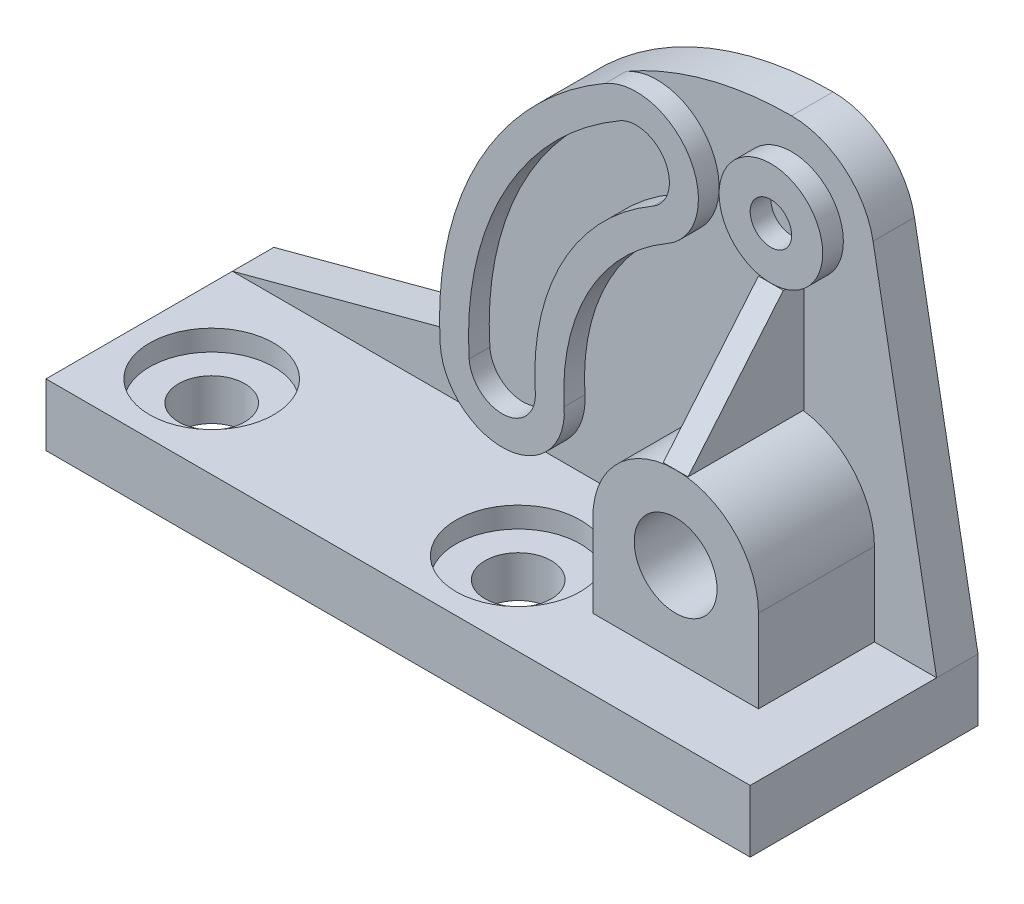
ISO-10303-21;
HEADER;
FILE_DESCRIPTION(('STEP AP214'),'2;1');
FILE_NAME('part.step','',(''),(''),'','','');
FILE_SCHEMA(('AUTOMOTIVE_DESIGN { 1 0 10303 214 1 1 1 1 }'));
ENDSEC;
DATA;
#1=APPLICATION_CONTEXT('core data for automotive mechanical design processes');
#2=APPLICATION_PROTOCOL_DEFINITION('international standard','automotive_design',2000,#1);
#3=PRODUCT_CONTEXT('',#1,'mechanical');
#4=PRODUCT('Part','Part','',(#3));
#5=PRODUCT_RELATED_PRODUCT_CATEGORY('part','',(#4));
#6=PRODUCT_DEFINITION_FORMATION('','',#4);
#7=PRODUCT_DEFINITION_CONTEXT('part definition',#1,'design');
#8=PRODUCT_DEFINITION('design','',#6,#7);
#9=PRODUCT_DEFINITION_SHAPE('','',#8);
#10=(LENGTH_UNIT() NAMED_UNIT(*) SI_UNIT(.MILLI.,.METRE.));
#11=(NAMED_UNIT(*) PLANE_ANGLE_UNIT() SI_UNIT($,.RADIAN.));
#12=(NAMED_UNIT(*) SI_UNIT($,.STERADIAN.) SOLID_ANGLE_UNIT());
#13=UNCERTAINTY_MEASURE_WITH_UNIT(LENGTH_MEASURE(1.E-05),#10,'distance_accuracy_value','');
#14=(GEOMETRIC_REPRESENTATION_CONTEXT(3) GLOBAL_UNCERTAINTY_ASSIGNED_CONTEXT((#13)) GLOBAL_UNIT_ASSIGNED_CONTEXT((#10,
#11,#12)) REPRESENTATION_CONTEXT('',''));
#15=CARTESIAN_POINT('',(0.,0.,0.));
#16=DIRECTION('',(0.,0.,1.));
#17=DIRECTION('',(1.,0.,0.));
#18=AXIS2_PLACEMENT_3D('',#15,#16,#17);
#19=CARTESIAN_POINT('',(26.5,41.25,-6.25));
#20=DIRECTION('',(0.,-1.,0.));
#21=DIRECTION('',(0.,0.,-1.));
#22=AXIS2_PLACEMENT_3D('',#19,#20,#21);
#23=PLANE('',#22);
#24=DIRECTION('',(0.,0.,1.));
#25=VECTOR('',#24,1.);
#26=CARTESIAN_POINT('',(23.5,41.25,-6.25));
#27=LINE('',#26,#25);
#28=CARTESIAN_POINT('',(23.5,41.25,-8.75));
#29=VERTEX_POINT('',#28);
#30=CARTESIAN_POINT('',(23.5,41.25,-6.25));
#31=VERTEX_POINT('',#30);
#32=EDGE_CURVE('E115',#29,#31,#27,.T.);
#33=ORIENTED_EDGE('',*,*,#32,.T.);
#34=DIRECTION('',(-1.,0.,0.));
#35=VECTOR('',#34,1.);
#36=CARTESIAN_POINT('',(26.5,41.25,-6.25));
#37=LINE('',#36,#35);
#38=CARTESIAN_POINT('',(26.5,41.25,-6.25));
#39=VERTEX_POINT('',#38);
#40=EDGE_CURVE('E12',#39,#31,#37,.T.);
#41=ORIENTED_EDGE('',*,*,#40,.F.);
#42=DIRECTION('',(0.,0.,1.));
#43=VECTOR('',#42,1.);
#44=CARTESIAN_POINT('',(26.5,41.25,-6.25));
#45=LINE('',#44,#43);
#46=CARTESIAN_POINT('',(26.5,41.25,-8.75));
#47=VERTEX_POINT('',#46);
#48=EDGE_CURVE('E99',#47,#39,#45,.T.);
#49=ORIENTED_EDGE('',*,*,#48,.F.);
#50=DIRECTION('',(-1.,0.,0.));
#51=VECTOR('',#50,1.);
#52=CARTESIAN_POINT('',(26.5,41.25,-8.75));
#53=LINE('',#52,#51);
#54=EDGE_CURVE('E107',#47,#29,#53,.T.);
#55=ORIENTED_EDGE('',*,*,#54,.T.);
#56=EDGE_LOOP('',(#33,#41,#49,#55));
#57=FACE_BOUND('',#56,.T.);
#58=ADVANCED_FACE('F47',(#57),#23,.F.);
#59=CARTESIAN_POINT('',(26.5,41.25,-6.25));
#60=DIRECTION('',(0.,-0.641555200491106,-0.767076870152409));
#61=DIRECTION('',(0.,0.767076870152409,-0.641555200491106));
#62=AXIS2_PLACEMENT_3D('',#59,#60,#61);
#63=PLANE('',#62);
#64=DIRECTION('',(0.,-0.767076870152409,0.641555200491106));
#65=VECTOR('',#64,1.);
#66=CARTESIAN_POINT('',(23.5,41.25,-6.25));
#67=LINE('',#66,#65);
#68=CARTESIAN_POINT('',(23.5,27.5,5.25));
#69=VERTEX_POINT('',#68);
#70=EDGE_CURVE('E102',#31,#69,#67,.T.);
#71=ORIENTED_EDGE('',*,*,#70,.T.);
#72=DIRECTION('',(-1.,0.,0.));
#73=VECTOR('',#72,1.);
#74=CARTESIAN_POINT('',(26.5,27.5,5.25));
#75=LINE('',#74,#73);
#76=CARTESIAN_POINT('',(26.5,27.5,5.25));
#77=VERTEX_POINT('',#76);
#78=EDGE_CURVE('E60',#77,#69,#75,.T.);
#79=ORIENTED_EDGE('',*,*,#78,.F.);
#80=DIRECTION('',(0.,-0.767076870152409,0.641555200491106));
#81=VECTOR('',#80,1.);
#82=CARTESIAN_POINT('',(26.5,41.25,-6.25));
#83=LINE('',#82,#81);
#84=EDGE_CURVE('E92',#39,#77,#83,.T.);
#85=ORIENTED_EDGE('',*,*,#84,.F.);
#86=ORIENTED_EDGE('',*,*,#40,.T.);
#87=EDGE_LOOP('',(#71,#79,#85,#86));
#88=FACE_BOUND('',#87,.T.);
#89=ADVANCED_FACE('F103',(#88),#63,.F.);
#90=CARTESIAN_POINT('',(26.5,27.5,-8.75));
#91=DIRECTION('',(0.,1.,0.));
#92=DIRECTION('',(0.,0.,1.));
#93=AXIS2_PLACEMENT_3D('',#90,#91,#92);
#94=PLANE('',#93);
#95=DIRECTION('',(0.,0.,-1.));
#96=VECTOR('',#95,1.);
#97=CARTESIAN_POINT('',(23.5,27.5,-8.75));
#98=LINE('',#97,#96);
#99=CARTESIAN_POINT('',(23.5,27.5,-8.75));
#100=VERTEX_POINT('',#99);
#101=EDGE_CURVE('E85',#69,#100,#98,.T.);
#102=ORIENTED_EDGE('',*,*,#101,.T.);
#103=DIRECTION('',(-1.,0.,0.));
#104=VECTOR('',#103,1.);
#105=CARTESIAN_POINT('',(26.5,27.5,-8.75));
#106=LINE('',#105,#104);
#107=CARTESIAN_POINT('',(26.5,27.5,-8.75));
#108=VERTEX_POINT('',#107);
#109=EDGE_CURVE('E104',#108,#100,#106,.T.);
#110=ORIENTED_EDGE('',*,*,#109,.F.);
#111=DIRECTION('',(0.,0.,-1.));
#112=VECTOR('',#111,1.);
#113=CARTESIAN_POINT('',(26.5,27.5,-8.75));
#114=LINE('',#113,#112);
#115=EDGE_CURVE('E98',#77,#108,#114,.T.);
#116=ORIENTED_EDGE('',*,*,#115,.F.);
#117=ORIENTED_EDGE('',*,*,#78,.T.);
#118=EDGE_LOOP('',(#102,#110,#116,#117));
#119=FACE_BOUND('',#118,.T.);
#120=ADVANCED_FACE('F106',(#119),#94,.F.);
#121=CARTESIAN_POINT('',(26.5,41.25,-8.75));
#122=DIRECTION('',(0.,0.,1.));
#123=DIRECTION('',(1.,0.,0.));
#124=AXIS2_PLACEMENT_3D('',#121,#122,#123);
#125=PLANE('',#124);
#126=DIRECTION('',(0.,1.,0.));
#127=VECTOR('',#126,1.);
#128=CARTESIAN_POINT('',(23.5,41.25,-8.75));
#129=LINE('',#128,#127);
#130=EDGE_CURVE('E86',#100,#29,#129,.T.);
#131=ORIENTED_EDGE('',*,*,#130,.T.);
#132=ORIENTED_EDGE('',*,*,#54,.F.);
#133=DIRECTION('',(0.,1.,0.));
#134=VECTOR('',#133,1.);
#135=CARTESIAN_POINT('',(26.5,41.25,-8.75));
#136=LINE('',#135,#134);
#137=EDGE_CURVE('E65',#108,#47,#136,.T.);
#138=ORIENTED_EDGE('',*,*,#137,.F.);
#139=ORIENTED_EDGE('',*,*,#109,.T.);
#140=EDGE_LOOP('',(#131,#132,#138,#139));
#141=FACE_BOUND('',#140,.T.);
#142=ADVANCED_FACE('F118',(#141),#125,.F.);
#143=CARTESIAN_POINT('',(26.5,0.,0.));
#144=DIRECTION('',(-1.,0.,0.));
#145=DIRECTION('',(0.,0.,1.));
#146=AXIS2_PLACEMENT_3D('',#143,#144,#145);
#147=PLANE('',#146);
#148=ORIENTED_EDGE('',*,*,#48,.T.);
#149=ORIENTED_EDGE('',*,*,#84,.T.);
#150=ORIENTED_EDGE('',*,*,#115,.T.);
#151=ORIENTED_EDGE('',*,*,#137,.T.);
#152=EDGE_LOOP('',(#148,#149,#150,#151));
#153=FACE_BOUND('',#152,.T.);
#154=ADVANCED_FACE('F96',(#153),#147,.F.);
#155=CARTESIAN_POINT('',(23.5,0.,0.));
#156=DIRECTION('',(-1.,0.,0.));
#157=DIRECTION('',(0.,0.,1.));
#158=AXIS2_PLACEMENT_3D('',#155,#156,#157);
#159=PLANE('',#158);
#160=ORIENTED_EDGE('',*,*,#32,.F.);
#161=ORIENTED_EDGE('',*,*,#130,.F.);
#162=ORIENTED_EDGE('',*,*,#101,.F.);
#163=ORIENTED_EDGE('',*,*,#70,.F.);
#164=EDGE_LOOP('',(#160,#161,#162,#163));
#165=FACE_BOUND('',#164,.T.);
#166=ADVANCED_FACE('F125',(#165),#159,.T.);
#167=CLOSED_SHELL('',(#58,#89,#120,#142,#154,#166));
#168=MANIFOLD_SOLID_BREP('B2',#167);
#169=CARTESIAN_POINT('',(25.,17.5,-8.75));
#170=DIRECTION('',(0.,0.,1.));
#171=DIRECTION('',(1.,0.,0.));
#172=AXIS2_PLACEMENT_3D('',#169,#170,#171);
#173=PLANE('',#172);
#174=CARTESIAN_POINT('',(25.,47.5,-8.75));
#175=DIRECTION('',(0.,0.,1.));
#176=DIRECTION('',(1.,0.,0.));
#177=AXIS2_PLACEMENT_3D('',#174,#175,#176);
#178=CIRCLE('',#177,6.25);
#179=CARTESIAN_POINT('',(31.25,47.5,-8.75));
#180=VERTEX_POINT('',#179);
#181=EDGE_CURVE('E430',#180,#180,#178,.T.);
#182=ORIENTED_EDGE('',*,*,#181,.F.);
#183=EDGE_LOOP('',(#182));
#184=FACE_BOUND('',#183,.T.);
#185=CARTESIAN_POINT('',(25.,17.5,-8.75));
#186=DIRECTION('',(0.,0.,-1.));
#187=DIRECTION('',(1.,0.,0.));
#188=AXIS2_PLACEMENT_3D('',#185,#186,#187);
#189=CIRCLE('',#188,40.);
#190=CARTESIAN_POINT('',(5.00000000000002,52.1410161513775,-8.75));
#191=VERTEX_POINT('',#190);
#192=CARTESIAN_POINT('',(25.,57.5,-8.75));
#193=VERTEX_POINT('',#192);
#194=EDGE_CURVE('E432',#191,#193,#189,.T.);
#195=ORIENTED_EDGE('',*,*,#194,.F.);
#196=CARTESIAN_POINT('',(8.74999999999999,45.6458256229943,-8.75));
#197=DIRECTION('',(0.,0.,1.));
#198=DIRECTION('',(-1.,0.,0.));
#199=AXIS2_PLACEMENT_3D('',#196,#197,#198);
#200=CIRCLE('',#199,7.49999999999999);
#201=CARTESIAN_POINT('',(12.5,39.1506350946109,-8.75));
#202=VERTEX_POINT('',#201);
#203=EDGE_CURVE('E326',#202,#191,#200,.T.);
#204=ORIENTED_EDGE('',*,*,#203,.F.);
#205=CARTESIAN_POINT('',(25.,17.5,-8.75));
#206=DIRECTION('',(0.,0.,-1.));
#207=DIRECTION('',(1.,0.,0.));
#208=AXIS2_PLACEMENT_3D('',#205,#206,#207);
#209=CIRCLE('',#208,25.);
#210=CARTESIAN_POINT('',(0.0532183429704687,15.8696365569313,-8.75));
#211=VERTEX_POINT('',#210);
#212=EDGE_CURVE('E352',#211,#202,#209,.T.);
#213=ORIENTED_EDGE('',*,*,#212,.F.);
#214=CARTESIAN_POINT('',(-7.4308161541384,15.3805275240106,-8.75));
#215=DIRECTION('',(0.,0.,1.));
#216=DIRECTION('',(1.,0.,0.));
#217=AXIS2_PLACEMENT_3D('',#214,#215,#216);
#218=CIRCLE('',#217,7.5);
#219=CARTESIAN_POINT('',(-14.9148506512472,14.89141849109,-8.75));
#220=VERTEX_POINT('',#219);
#221=EDGE_CURVE('E363',#220,#211,#218,.T.);
#222=ORIENTED_EDGE('',*,*,#221,.F.);
#223=DIRECTION('',(0.96592582628907,0.258819045102514,0.));
#224=VECTOR('',#223,1.);
#225=CARTESIAN_POINT('',(-42.5,7.5,-8.75));
#226=LINE('',#225,#224);
#227=CARTESIAN_POINT('',(-42.5,7.5,-8.75));
#228=VERTEX_POINT('',#227);
#229=EDGE_CURVE('E447',#228,#220,#226,.T.);
#230=ORIENTED_EDGE('',*,*,#229,.F.);
#231=DIRECTION('',(-1.,0.,0.));
#232=VECTOR('',#231,1.);
#233=CARTESIAN_POINT('',(42.5,7.5,-8.75));
#234=LINE('',#233,#232);
#235=CARTESIAN_POINT('',(15.,7.5,-8.75));
#236=VERTEX_POINT('',#235);
#237=EDGE_CURVE('E444',#236,#228,#234,.T.);
#238=ORIENTED_EDGE('',*,*,#237,.F.);
#239=DIRECTION('',(0.,-1.,0.));
#240=VECTOR('',#239,1.);
#241=CARTESIAN_POINT('',(15.,17.5,-8.75));
#242=LINE('',#241,#240);
#243=CARTESIAN_POINT('',(15.,17.5,-8.75));
#244=VERTEX_POINT('',#243);
#245=EDGE_CURVE('E415',#244,#236,#242,.T.);
#246=ORIENTED_EDGE('',*,*,#245,.F.);
#247=CARTESIAN_POINT('',(25.,17.5,-8.75));
#248=DIRECTION('',(0.,0.,1.));
#249=DIRECTION('',(1.,0.,0.));
#250=AXIS2_PLACEMENT_3D('',#247,#248,#249);
#251=CIRCLE('',#250,10.);
#252=CARTESIAN_POINT('',(35.,17.5,-8.75));
#253=VERTEX_POINT('',#252);
#254=EDGE_CURVE('E397',#253,#244,#251,.T.);
#255=ORIENTED_EDGE('',*,*,#254,.F.);
#256=DIRECTION('',(0.,1.,0.));
#257=VECTOR('',#256,1.);
#258=CARTESIAN_POINT('',(35.,7.5,-8.75));
#259=LINE('',#258,#257);
#260=CARTESIAN_POINT('',(35.,7.5,-8.75));
#261=VERTEX_POINT('',#260);
#262=EDGE_CURVE('E401',#261,#253,#259,.T.);
#263=ORIENTED_EDGE('',*,*,#262,.F.);
#264=CARTESIAN_POINT('',(42.5,7.5,-8.75));
#265=VERTEX_POINT('',#264);
#266=EDGE_CURVE('E441',#265,#261,#234,.T.);
#267=ORIENTED_EDGE('',*,*,#266,.F.);
#268=DIRECTION('',(0.180327868852459,-0.983606557377049,0.));
#269=VECTOR('',#268,1.);
#270=CARTESIAN_POINT('',(34.8360655737705,49.3032786885246,-8.75));
#271=LINE('',#270,#269);
#272=CARTESIAN_POINT('',(34.8360655737705,49.3032786885246,-8.75));
#273=VERTEX_POINT('',#272);
#274=EDGE_CURVE('E439',#273,#265,#271,.T.);
#275=ORIENTED_EDGE('',*,*,#274,.F.);
#276=CARTESIAN_POINT('',(25.,47.5,-8.75));
#277=DIRECTION('',(0.,0.,-1.));
#278=DIRECTION('',(-1.,0.,0.));
#279=AXIS2_PLACEMENT_3D('',#276,#277,#278);
#280=CIRCLE('',#279,10.);
#281=EDGE_CURVE('E436',#193,#273,#280,.T.);
#282=ORIENTED_EDGE('',*,*,#281,.F.);
#283=EDGE_LOOP('',(#195,#204,#213,#222,#230,#238,#246,#255,#263,#267,#275,#282));
#284=FACE_BOUND('',#283,.T.);
#285=ADVANCED_FACE('F174',(#184,#284),#173,.T.);
#286=CARTESIAN_POINT('',(0.,7.5,0.));
#287=DIRECTION('',(0.,-1.,0.));
#288=DIRECTION('',(0.,0.,-1.));
#289=AXIS2_PLACEMENT_3D('',#286,#287,#288);
#290=PLANE('',#289);
#291=CARTESIAN_POINT('',(4.5,7.5,3.75));
#292=DIRECTION('',(0.,1.,0.));
#293=DIRECTION('',(0.,0.,1.));
#294=AXIS2_PLACEMENT_3D('',#291,#292,#293);
#295=CIRCLE('',#294,7.5);
#296=CARTESIAN_POINT('',(4.5,7.5,11.25));
#297=VERTEX_POINT('',#296);
#298=EDGE_CURVE('E389',#297,#297,#295,.T.);
#299=ORIENTED_EDGE('',*,*,#298,.F.);
#300=EDGE_LOOP('',(#299));
#301=FACE_BOUND('',#300,.T.);
#302=CARTESIAN_POINT('',(-32.5,7.5,3.75));
#303=DIRECTION('',(0.,1.,0.));
#304=DIRECTION('',(0.,0.,1.));
#305=AXIS2_PLACEMENT_3D('',#302,#303,#304);
#306=CIRCLE('',#305,7.5);
#307=CARTESIAN_POINT('',(-32.5,7.5,11.25));
#308=VERTEX_POINT('',#307);
#309=EDGE_CURVE('E374',#308,#308,#306,.T.);
#310=ORIENTED_EDGE('',*,*,#309,.F.);
#311=EDGE_LOOP('',(#310));
#312=FACE_BOUND('',#311,.T.);
#313=DIRECTION('',(0.,0.,-1.));
#314=VECTOR('',#313,1.);
#315=CARTESIAN_POINT('',(15.,7.5,5.25));
#316=LINE('',#315,#314);
#317=CARTESIAN_POINT('',(15.,7.5,5.25));
#318=VERTEX_POINT('',#317);
#319=EDGE_CURVE('E420',#318,#236,#316,.T.);
#320=ORIENTED_EDGE('',*,*,#319,.T.);
#321=ORIENTED_EDGE('',*,*,#237,.T.);
#322=DIRECTION('',(0.,0.,1.));
#323=VECTOR('',#322,1.);
#324=CARTESIAN_POINT('',(-42.5,7.5,13.75));
#325=LINE('',#324,#323);
#326=CARTESIAN_POINT('',(-42.5,7.5,13.75));
#327=VERTEX_POINT('',#326);
#328=EDGE_CURVE('E472',#228,#327,#325,.T.);
#329=ORIENTED_EDGE('',*,*,#328,.T.);
#330=DIRECTION('',(1.,0.,0.));
#331=VECTOR('',#330,1.);
#332=CARTESIAN_POINT('',(-42.5,7.5,13.75));
#333=LINE('',#332,#331);
#334=CARTESIAN_POINT('',(42.5,7.5,13.75));
#335=VERTEX_POINT('',#334);
#336=EDGE_CURVE('E480',#327,#335,#333,.T.);
#337=ORIENTED_EDGE('',*,*,#336,.T.);
#338=DIRECTION('',(0.,0.,-1.));
#339=VECTOR('',#338,1.);
#340=CARTESIAN_POINT('',(42.5,7.5,13.75));
#341=LINE('',#340,#339);
#342=EDGE_CURVE('E468',#335,#265,#341,.T.);
#343=ORIENTED_EDGE('',*,*,#342,.T.);
#344=ORIENTED_EDGE('',*,*,#266,.T.);
#345=DIRECTION('',(0.,0.,-1.));
#346=VECTOR('',#345,1.);
#347=CARTESIAN_POINT('',(35.,7.5,5.25));
#348=LINE('',#347,#346);
#349=CARTESIAN_POINT('',(35.,7.5,5.25));
#350=VERTEX_POINT('',#349);
#351=EDGE_CURVE('E417',#350,#261,#348,.T.);
#352=ORIENTED_EDGE('',*,*,#351,.F.);
#353=DIRECTION('',(1.,0.,0.));
#354=VECTOR('',#353,1.);
#355=CARTESIAN_POINT('',(15.,7.5,5.25));
#356=LINE('',#355,#354);
#357=EDGE_CURVE('E403',#318,#350,#356,.T.);
#358=ORIENTED_EDGE('',*,*,#357,.F.);
#359=EDGE_LOOP('',(#320,#321,#329,#337,#343,#344,#352,#358));
#360=FACE_BOUND('',#359,.T.);
#361=ADVANCED_FACE('F527',(#301,#312,#360),#290,.F.);
#362=CARTESIAN_POINT('',(42.5,7.5,13.75));
#363=DIRECTION('',(-1.,0.,0.));
#364=DIRECTION('',(0.,0.,1.));
#365=AXIS2_PLACEMENT_3D('',#362,#363,#364);
#366=PLANE('',#365);
#367=DIRECTION('',(0.,0.,-1.));
#368=VECTOR('',#367,1.);
#369=CARTESIAN_POINT('',(42.5,0.,13.75));
#370=LINE('',#369,#368);
#371=CARTESIAN_POINT('',(42.5,0.,13.75));
#372=VERTEX_POINT('',#371);
#373=CARTESIAN_POINT('',(42.5,0.,-13.75));
#374=VERTEX_POINT('',#373);
#375=EDGE_CURVE('E464',#372,#374,#370,.T.);
#376=ORIENTED_EDGE('',*,*,#375,.T.);
#377=DIRECTION('',(0.,-1.,0.));
#378=VECTOR('',#377,1.);
#379=CARTESIAN_POINT('',(42.5,7.5,-13.75));
#380=LINE('',#379,#378);
#381=CARTESIAN_POINT('',(42.5,7.5,-13.75));
#382=VERTEX_POINT('',#381);
#383=EDGE_CURVE('E494',#382,#374,#380,.T.);
#384=ORIENTED_EDGE('',*,*,#383,.F.);
#385=DIRECTION('',(0.,0.,-1.));
#386=VECTOR('',#385,1.);
#387=CARTESIAN_POINT('',(42.5,7.5,-8.75));
#388=LINE('',#387,#386);
#389=EDGE_CURVE('E463',#265,#382,#388,.T.);
#390=ORIENTED_EDGE('',*,*,#389,.F.);
#391=ORIENTED_EDGE('',*,*,#342,.F.);
#392=DIRECTION('',(0.,-1.,0.));
#393=VECTOR('',#392,1.);
#394=CARTESIAN_POINT('',(42.5,7.5,13.75));
#395=LINE('',#394,#393);
#396=EDGE_CURVE('E479',#335,#372,#395,.T.);
#397=ORIENTED_EDGE('',*,*,#396,.T.);
#398=EDGE_LOOP('',(#376,#384,#390,#391,#397));
#399=FACE_BOUND('',#398,.T.);
#400=ADVANCED_FACE('F175',(#399),#366,.F.);
#401=CARTESIAN_POINT('',(-42.5,7.5,-13.75));
#402=DIRECTION('',(0.,0.,1.));
#403=DIRECTION('',(1.,0.,0.));
#404=AXIS2_PLACEMENT_3D('',#401,#402,#403);
#405=PLANE('',#404);
#406=DIRECTION('',(-1.,0.,0.));
#407=VECTOR('',#406,1.);
#408=CARTESIAN_POINT('',(-42.5,0.,-13.75));
#409=LINE('',#408,#407);
#410=CARTESIAN_POINT('',(-42.5,0.,-13.75));
#411=VERTEX_POINT('',#410);
#412=EDGE_CURVE('E485',#374,#411,#409,.T.);
#413=ORIENTED_EDGE('',*,*,#412,.T.);
#414=DIRECTION('',(0.,-1.,0.));
#415=VECTOR('',#414,1.);
#416=CARTESIAN_POINT('',(-42.5,7.5,-13.75));
#417=LINE('',#416,#415);
#418=CARTESIAN_POINT('',(-42.5,7.5,-13.75));
#419=VERTEX_POINT('',#418);
#420=EDGE_CURVE('E495',#419,#411,#417,.T.);
#421=ORIENTED_EDGE('',*,*,#420,.F.);
#422=DIRECTION('',(0.96592582628907,0.258819045102514,0.));
#423=VECTOR('',#422,1.);
#424=CARTESIAN_POINT('',(-42.5,7.5,-13.75));
#425=LINE('',#424,#423);
#426=CARTESIAN_POINT('',(-14.9148506512473,14.89141849109,-13.75));
#427=VERTEX_POINT('',#426);
#428=EDGE_CURVE('E440',#419,#427,#425,.T.);
#429=ORIENTED_EDGE('',*,*,#428,.T.);
#430=CARTESIAN_POINT('',(25.,17.5,-13.75));
#431=DIRECTION('',(0.,0.,-1.));
#432=DIRECTION('',(1.,0.,0.));
#433=AXIS2_PLACEMENT_3D('',#430,#431,#432);
#434=CIRCLE('',#433,40.);
#435=CARTESIAN_POINT('',(25.,57.5,-13.75));
#436=VERTEX_POINT('',#435);
#437=EDGE_CURVE('E431',#427,#436,#434,.T.);
#438=ORIENTED_EDGE('',*,*,#437,.T.);
#439=CARTESIAN_POINT('',(25.,47.5,-13.75));
#440=DIRECTION('',(0.,0.,-1.));
#441=DIRECTION('',(-1.,0.,0.));
#442=AXIS2_PLACEMENT_3D('',#439,#440,#441);
#443=CIRCLE('',#442,10.);
#444=CARTESIAN_POINT('',(34.8360655737705,49.3032786885246,-13.75));
#445=VERTEX_POINT('',#444);
#446=EDGE_CURVE('E452',#436,#445,#443,.T.);
#447=ORIENTED_EDGE('',*,*,#446,.T.);
#448=DIRECTION('',(0.180327868852459,-0.983606557377049,0.));
#449=VECTOR('',#448,1.);
#450=CARTESIAN_POINT('',(34.8360655737705,49.3032786885246,-13.75));
#451=LINE('',#450,#449);
#452=EDGE_CURVE('E457',#445,#382,#451,.T.);
#453=ORIENTED_EDGE('',*,*,#452,.T.);
#454=ORIENTED_EDGE('',*,*,#383,.T.);
#455=EDGE_LOOP('',(#413,#421,#429,#438,#447,#453,#454));
#456=FACE_BOUND('',#455,.T.);
#457=ADVANCED_FACE('F554',(#456),#405,.F.);
#458=CARTESIAN_POINT('',(-42.5,7.5,13.75));
#459=DIRECTION('',(1.,0.,0.));
#460=DIRECTION('',(0.,0.,-1.));
#461=AXIS2_PLACEMENT_3D('',#458,#459,#460);
#462=PLANE('',#461);
#463=DIRECTION('',(0.,0.,1.));
#464=VECTOR('',#463,1.);
#465=CARTESIAN_POINT('',(-42.5,0.,13.75));
#466=LINE('',#465,#464);
#467=CARTESIAN_POINT('',(-42.5,0.,13.75));
#468=VERTEX_POINT('',#467);
#469=EDGE_CURVE('E482',#411,#468,#466,.T.);
#470=ORIENTED_EDGE('',*,*,#469,.T.);
#471=DIRECTION('',(0.,-1.,0.));
#472=VECTOR('',#471,1.);
#473=CARTESIAN_POINT('',(-42.5,7.5,13.75));
#474=LINE('',#473,#472);
#475=EDGE_CURVE('E487',#327,#468,#474,.T.);
#476=ORIENTED_EDGE('',*,*,#475,.F.);
#477=ORIENTED_EDGE('',*,*,#328,.F.);
#478=EDGE_CURVE('E475',#419,#228,#325,.T.);
#479=ORIENTED_EDGE('',*,*,#478,.F.);
#480=ORIENTED_EDGE('',*,*,#420,.T.);
#481=EDGE_LOOP('',(#470,#476,#477,#479,#480));
#482=FACE_BOUND('',#481,.T.);
#483=ADVANCED_FACE('F847',(#482),#462,.F.);
#484=CARTESIAN_POINT('',(-42.5,7.5,13.75));
#485=DIRECTION('',(0.,0.,-1.));
#486=DIRECTION('',(-1.,0.,0.));
#487=AXIS2_PLACEMENT_3D('',#484,#485,#486);
#488=PLANE('',#487);
#489=DIRECTION('',(1.,0.,0.));
#490=VECTOR('',#489,1.);
#491=CARTESIAN_POINT('',(-42.5,0.,13.75));
#492=LINE('',#491,#490);
#493=EDGE_CURVE('E471',#468,#372,#492,.T.);
#494=ORIENTED_EDGE('',*,*,#493,.T.);
#495=ORIENTED_EDGE('',*,*,#396,.F.);
#496=ORIENTED_EDGE('',*,*,#336,.F.);
#497=ORIENTED_EDGE('',*,*,#475,.T.);
#498=EDGE_LOOP('',(#494,#495,#496,#497));
#499=FACE_BOUND('',#498,.T.);
#500=ADVANCED_FACE('F837',(#499),#488,.F.);
#501=CARTESIAN_POINT('',(0.,0.,0.));
#502=DIRECTION('',(0.,-1.,0.));
#503=DIRECTION('',(0.,0.,-1.));
#504=AXIS2_PLACEMENT_3D('',#501,#502,#503);
#505=PLANE('',#504);
#506=CARTESIAN_POINT('',(-32.5,0.,3.75));
#507=DIRECTION('',(0.,1.,0.));
#508=DIRECTION('',(0.,0.,1.));
#509=AXIS2_PLACEMENT_3D('',#506,#507,#508);
#510=CIRCLE('',#509,4.);
#511=CARTESIAN_POINT('',(-32.5,0.,7.75));
#512=VERTEX_POINT('',#511);
#513=EDGE_CURVE('E375',#512,#512,#510,.T.);
#514=ORIENTED_EDGE('',*,*,#513,.T.);
#515=EDGE_LOOP('',(#514));
#516=FACE_BOUND('',#515,.T.);
#517=CARTESIAN_POINT('',(4.5,0.,3.75));
#518=DIRECTION('',(0.,1.,0.));
#519=DIRECTION('',(0.,0.,1.));
#520=AXIS2_PLACEMENT_3D('',#517,#518,#519);
#521=CIRCLE('',#520,4.);
#522=CARTESIAN_POINT('',(4.5,0.,7.75));
#523=VERTEX_POINT('',#522);
#524=EDGE_CURVE('E377',#523,#523,#521,.T.);
#525=ORIENTED_EDGE('',*,*,#524,.T.);
#526=EDGE_LOOP('',(#525));
#527=FACE_BOUND('',#526,.T.);
#528=ORIENTED_EDGE('',*,*,#375,.F.);
#529=ORIENTED_EDGE('',*,*,#493,.F.);
#530=ORIENTED_EDGE('',*,*,#469,.F.);
#531=ORIENTED_EDGE('',*,*,#412,.F.);
#532=EDGE_LOOP('',(#528,#529,#530,#531));
#533=FACE_BOUND('',#532,.T.);
#534=ADVANCED_FACE('F735',(#516,#527,#533),#505,.T.);
#535=CARTESIAN_POINT('',(25.,17.5,-8.75));
#536=DIRECTION('',(0.,0.,-1.));
#537=DIRECTION('',(-1.,0.,0.));
#538=AXIS2_PLACEMENT_3D('',#535,#536,#537);
#539=CYLINDRICAL_SURFACE('',#538,40.);
#540=ORIENTED_EDGE('',*,*,#437,.F.);
#541=DIRECTION('',(0.,0.,-1.));
#542=VECTOR('',#541,1.);
#543=CARTESIAN_POINT('',(-14.9148506512473,14.89141849109,-8.75));
#544=LINE('',#543,#542);
#545=EDGE_CURVE('E461',#220,#427,#544,.T.);
#546=ORIENTED_EDGE('',*,*,#545,.F.);
#547=DIRECTION('',(0.,0.,-1.));
#548=VECTOR('',#547,1.);
#549=CARTESIAN_POINT('',(-14.9148506512472,14.89141849109,-6.25));
#550=LINE('',#549,#548);
#551=CARTESIAN_POINT('',(-14.9148506512472,14.89141849109,-6.25));
#552=VERTEX_POINT('',#551);
#553=EDGE_CURVE('E370',#552,#220,#550,.T.);
#554=ORIENTED_EDGE('',*,*,#553,.F.);
#555=CARTESIAN_POINT('',(25.,17.5,-6.25));
#556=DIRECTION('',(0.,0.,1.));
#557=DIRECTION('',(1.,0.,0.));
#558=AXIS2_PLACEMENT_3D('',#555,#556,#557);
#559=CIRCLE('',#558,40.);
#560=CARTESIAN_POINT('',(5.00000000000002,52.1410161513775,-6.25));
#561=VERTEX_POINT('',#560);
#562=EDGE_CURVE('E351',#561,#552,#559,.T.);
#563=ORIENTED_EDGE('',*,*,#562,.F.);
#564=DIRECTION('',(0.,0.,-1.));
#565=VECTOR('',#564,1.);
#566=CARTESIAN_POINT('',(5.00000000000002,52.1410161513775,-6.25));
#567=LINE('',#566,#565);
#568=EDGE_CURVE('E369',#561,#191,#567,.T.);
#569=ORIENTED_EDGE('',*,*,#568,.T.);
#570=ORIENTED_EDGE('',*,*,#194,.T.);
#571=DIRECTION('',(0.,0.,-1.));
#572=VECTOR('',#571,1.);
#573=CARTESIAN_POINT('',(25.,57.5,-8.75));
#574=LINE('',#573,#572);
#575=EDGE_CURVE('E450',#193,#436,#574,.T.);
#576=ORIENTED_EDGE('',*,*,#575,.T.);
#577=EDGE_LOOP('',(#540,#546,#554,#563,#569,#570,#576));
#578=FACE_BOUND('',#577,.T.);
#579=ADVANCED_FACE('F546',(#578),#539,.T.);
#580=CARTESIAN_POINT('',(-42.5,7.5,-8.75));
#581=DIRECTION('',(-0.258819045102514,0.96592582628907,0.));
#582=DIRECTION('',(-0.96592582628907,-0.258819045102514,0.));
#583=AXIS2_PLACEMENT_3D('',#580,#581,#582);
#584=PLANE('',#583);
#585=ORIENTED_EDGE('',*,*,#428,.F.);
#586=ORIENTED_EDGE('',*,*,#478,.T.);
#587=ORIENTED_EDGE('',*,*,#229,.T.);
#588=ORIENTED_EDGE('',*,*,#545,.T.);
#589=EDGE_LOOP('',(#585,#586,#587,#588));
#590=FACE_BOUND('',#589,.T.);
#591=ADVANCED_FACE('F560',(#590),#584,.T.);
#592=CARTESIAN_POINT('',(34.8360655737705,49.3032786885246,-8.75));
#593=DIRECTION('',(0.983606557377049,0.180327868852459,0.));
#594=DIRECTION('',(-0.180327868852459,0.983606557377049,0.));
#595=AXIS2_PLACEMENT_3D('',#592,#593,#594);
#596=PLANE('',#595);
#597=ORIENTED_EDGE('',*,*,#452,.F.);
#598=DIRECTION('',(0.,0.,-1.));
#599=VECTOR('',#598,1.);
#600=CARTESIAN_POINT('',(34.8360655737705,49.3032786885246,-8.75));
#601=LINE('',#600,#599);
#602=EDGE_CURVE('E466',#273,#445,#601,.T.);
#603=ORIENTED_EDGE('',*,*,#602,.F.);
#604=ORIENTED_EDGE('',*,*,#274,.T.);
#605=ORIENTED_EDGE('',*,*,#389,.T.);
#606=EDGE_LOOP('',(#597,#603,#604,#605));
#607=FACE_BOUND('',#606,.T.);
#608=ADVANCED_FACE('F814',(#607),#596,.T.);
#609=CARTESIAN_POINT('',(25.,47.5,-8.75));
#610=DIRECTION('',(0.,0.,-1.));
#611=DIRECTION('',(-1.,0.,0.));
#612=AXIS2_PLACEMENT_3D('',#609,#610,#611);
#613=CYLINDRICAL_SURFACE('',#612,10.);
#614=ORIENTED_EDGE('',*,*,#446,.F.);
#615=ORIENTED_EDGE('',*,*,#575,.F.);
#616=ORIENTED_EDGE('',*,*,#281,.T.);
#617=ORIENTED_EDGE('',*,*,#602,.T.);
#618=EDGE_LOOP('',(#614,#615,#616,#617));
#619=FACE_BOUND('',#618,.T.);
#620=ADVANCED_FACE('F549',(#619),#613,.T.);
#621=CARTESIAN_POINT('',(25.,47.5,-6.25));
#622=DIRECTION('',(0.,0.,1.));
#623=DIRECTION('',(1.,0.,0.));
#624=AXIS2_PLACEMENT_3D('',#621,#622,#623);
#625=PLANE('',#624);
#626=CARTESIAN_POINT('',(25.,47.5,-6.25));
#627=DIRECTION('',(0.,0.,1.));
#628=DIRECTION('',(1.,0.,0.));
#629=AXIS2_PLACEMENT_3D('',#626,#627,#628);
#630=CIRCLE('',#629,6.25);
#631=CARTESIAN_POINT('',(31.25,47.5,-6.25));
#632=VERTEX_POINT('',#631);
#633=EDGE_CURVE('E428',#632,#632,#630,.T.);
#634=ORIENTED_EDGE('',*,*,#633,.T.);
#635=EDGE_LOOP('',(#634));
#636=FACE_BOUND('',#635,.T.);
#637=CARTESIAN_POINT('',(25.,47.5,-6.25));
#638=DIRECTION('',(0.,0.,1.));
#639=DIRECTION('',(1.,0.,0.));
#640=AXIS2_PLACEMENT_3D('',#637,#638,#639);
#641=CIRCLE('',#640,2.5);
#642=CARTESIAN_POINT('',(27.5,47.5,-6.25));
#643=VERTEX_POINT('',#642);
#644=EDGE_CURVE('E424',#643,#643,#641,.T.);
#645=ORIENTED_EDGE('',*,*,#644,.F.);
#646=EDGE_LOOP('',(#645));
#647=FACE_BOUND('',#646,.T.);
#648=ADVANCED_FACE('F625',(#636,#647),#625,.T.);
#649=CARTESIAN_POINT('',(25.,47.5,-6.25));
#650=DIRECTION('',(0.,0.,-1.));
#651=DIRECTION('',(-1.,0.,0.));
#652=AXIS2_PLACEMENT_3D('',#649,#650,#651);
#653=CYLINDRICAL_SURFACE('',#652,6.25);
#654=ORIENTED_EDGE('',*,*,#633,.F.);
#655=EDGE_LOOP('',(#654));
#656=FACE_BOUND('',#655,.T.);
#657=ORIENTED_EDGE('',*,*,#181,.T.);
#658=EDGE_LOOP('',(#657));
#659=FACE_BOUND('',#658,.T.);
#660=ADVANCED_FACE('F513',(#656,#659),#653,.T.);
#661=CARTESIAN_POINT('',(25.,47.5,-6.25));
#662=DIRECTION('',(0.,0.,-1.));
#663=DIRECTION('',(-1.,0.,0.));
#664=AXIS2_PLACEMENT_3D('',#661,#662,#663);
#665=CYLINDRICAL_SURFACE('',#664,2.5);
#666=ORIENTED_EDGE('',*,*,#644,.T.);
#667=EDGE_LOOP('',(#666));
#668=FACE_BOUND('',#667,.T.);
#669=CARTESIAN_POINT('',(25.,47.5,-8.75));
#670=DIRECTION('',(0.,0.,1.));
#671=DIRECTION('',(1.,0.,0.));
#672=AXIS2_PLACEMENT_3D('',#669,#670,#671);
#673=CIRCLE('',#672,2.5);
#674=CARTESIAN_POINT('',(27.5,47.5,-8.75));
#675=VERTEX_POINT('',#674);
#676=EDGE_CURVE('E182',#675,#675,#673,.F.);
#677=ORIENTED_EDGE('',*,*,#676,.T.);
#678=EDGE_LOOP('',(#677));
#679=FACE_BOUND('',#678,.T.);
#680=ADVANCED_FACE('F498',(#668,#679),#665,.F.);
#681=ORIENTED_EDGE('',*,*,#676,.F.);
#682=EDGE_LOOP('',(#681));
#683=FACE_BOUND('',#682,.T.);
#684=ADVANCED_FACE('F502',(#683),#173,.T.);
#685=CARTESIAN_POINT('',(25.,17.5,5.25));
#686=DIRECTION('',(0.,0.,1.));
#687=DIRECTION('',(1.,0.,0.));
#688=AXIS2_PLACEMENT_3D('',#685,#686,#687);
#689=PLANE('',#688);
#690=CARTESIAN_POINT('',(25.,17.5,5.25));
#691=DIRECTION('',(0.,0.,1.));
#692=DIRECTION('',(1.,0.,0.));
#693=AXIS2_PLACEMENT_3D('',#690,#691,#692);
#694=CIRCLE('',#693,10.);
#695=CARTESIAN_POINT('',(35.,17.5,5.25));
#696=VERTEX_POINT('',#695);
#697=CARTESIAN_POINT('',(15.,17.5,5.25));
#698=VERTEX_POINT('',#697);
#699=EDGE_CURVE('E398',#696,#698,#694,.T.);
#700=ORIENTED_EDGE('',*,*,#699,.T.);
#701=DIRECTION('',(0.,-1.,0.));
#702=VECTOR('',#701,1.);
#703=CARTESIAN_POINT('',(15.,17.5,5.25));
#704=LINE('',#703,#702);
#705=EDGE_CURVE('E405',#698,#318,#704,.T.);
#706=ORIENTED_EDGE('',*,*,#705,.T.);
#707=ORIENTED_EDGE('',*,*,#357,.T.);
#708=DIRECTION('',(0.,1.,0.));
#709=VECTOR('',#708,1.);
#710=CARTESIAN_POINT('',(35.,7.5,5.25));
#711=LINE('',#710,#709);
#712=EDGE_CURVE('E407',#350,#696,#711,.T.);
#713=ORIENTED_EDGE('',*,*,#712,.T.);
#714=EDGE_LOOP('',(#700,#706,#707,#713));
#715=FACE_BOUND('',#714,.T.);
#716=CARTESIAN_POINT('',(25.,17.5,5.25));
#717=DIRECTION('',(0.,0.,1.));
#718=DIRECTION('',(1.,0.,0.));
#719=AXIS2_PLACEMENT_3D('',#716,#717,#718);
#720=CIRCLE('',#719,5.);
#721=CARTESIAN_POINT('',(30.,17.5,5.25));
#722=VERTEX_POINT('',#721);
#723=EDGE_CURVE('E390',#722,#722,#720,.T.);
#724=ORIENTED_EDGE('',*,*,#723,.F.);
#725=EDGE_LOOP('',(#724));
#726=FACE_BOUND('',#725,.T.);
#727=ADVANCED_FACE('F503',(#715,#726),#689,.T.);
#728=CARTESIAN_POINT('',(25.,17.5,5.25));
#729=DIRECTION('',(0.,0.,-1.));
#730=DIRECTION('',(-1.,0.,0.));
#731=AXIS2_PLACEMENT_3D('',#728,#729,#730);
#732=CYLINDRICAL_SURFACE('',#731,10.);
#733=ORIENTED_EDGE('',*,*,#254,.T.);
#734=DIRECTION('',(0.,0.,-1.));
#735=VECTOR('',#734,1.);
#736=CARTESIAN_POINT('',(15.,17.5,5.25));
#737=LINE('',#736,#735);
#738=EDGE_CURVE('E425',#698,#244,#737,.T.);
#739=ORIENTED_EDGE('',*,*,#738,.F.);
#740=ORIENTED_EDGE('',*,*,#699,.F.);
#741=DIRECTION('',(0.,0.,-1.));
#742=VECTOR('',#741,1.);
#743=CARTESIAN_POINT('',(35.,17.5,5.25));
#744=LINE('',#743,#742);
#745=EDGE_CURVE('E408',#696,#253,#744,.T.);
#746=ORIENTED_EDGE('',*,*,#745,.T.);
#747=EDGE_LOOP('',(#733,#739,#740,#746));
#748=FACE_BOUND('',#747,.T.);
#749=ADVANCED_FACE('F515',(#748),#732,.T.);
#750=CARTESIAN_POINT('',(15.,17.5,5.25));
#751=DIRECTION('',(1.,0.,0.));
#752=DIRECTION('',(0.,0.,-1.));
#753=AXIS2_PLACEMENT_3D('',#750,#751,#752);
#754=PLANE('',#753);
#755=ORIENTED_EDGE('',*,*,#245,.T.);
#756=ORIENTED_EDGE('',*,*,#319,.F.);
#757=ORIENTED_EDGE('',*,*,#705,.F.);
#758=ORIENTED_EDGE('',*,*,#738,.T.);
#759=EDGE_LOOP('',(#755,#756,#757,#758));
#760=FACE_BOUND('',#759,.T.);
#761=ADVANCED_FACE('F613',(#760),#754,.F.);
#762=CARTESIAN_POINT('',(35.,7.5,5.25));
#763=DIRECTION('',(-1.,0.,0.));
#764=DIRECTION('',(0.,0.,1.));
#765=AXIS2_PLACEMENT_3D('',#762,#763,#764);
#766=PLANE('',#765);
#767=ORIENTED_EDGE('',*,*,#262,.T.);
#768=ORIENTED_EDGE('',*,*,#745,.F.);
#769=ORIENTED_EDGE('',*,*,#712,.F.);
#770=ORIENTED_EDGE('',*,*,#351,.T.);
#771=EDGE_LOOP('',(#767,#768,#769,#770));
#772=FACE_BOUND('',#771,.T.);
#773=ADVANCED_FACE('F606',(#772),#766,.F.);
#774=CARTESIAN_POINT('',(25.,17.5,5.25));
#775=DIRECTION('',(0.,0.,-1.));
#776=DIRECTION('',(-1.,0.,0.));
#777=AXIS2_PLACEMENT_3D('',#774,#775,#776);
#778=CYLINDRICAL_SURFACE('',#777,5.);
#779=ORIENTED_EDGE('',*,*,#723,.T.);
#780=EDGE_LOOP('',(#779));
#781=FACE_BOUND('',#780,.T.);
#782=CARTESIAN_POINT('',(25.,17.5,-8.75));
#783=DIRECTION('',(0.,0.,1.));
#784=DIRECTION('',(1.,0.,0.));
#785=AXIS2_PLACEMENT_3D('',#782,#783,#784);
#786=CIRCLE('',#785,5.);
#787=CARTESIAN_POINT('',(30.,17.5,-8.75));
#788=VERTEX_POINT('',#787);
#789=EDGE_CURVE('E50',#788,#788,#786,.F.);
#790=ORIENTED_EDGE('',*,*,#789,.T.);
#791=EDGE_LOOP('',(#790));
#792=FACE_BOUND('',#791,.T.);
#793=ADVANCED_FACE('F523',(#781,#792),#778,.F.);
#794=ORIENTED_EDGE('',*,*,#789,.F.);
#795=EDGE_LOOP('',(#794));
#796=FACE_BOUND('',#795,.T.);
#797=ADVANCED_FACE('F510',(#796),#173,.T.);
#798=CARTESIAN_POINT('',(-32.5,5.,3.75));
#799=DIRECTION('',(0.,1.,0.));
#800=DIRECTION('',(0.,0.,1.));
#801=AXIS2_PLACEMENT_3D('',#798,#799,#800);
#802=CYLINDRICAL_SURFACE('',#801,7.5);
#803=CARTESIAN_POINT('',(-32.5,5.,3.75));
#804=DIRECTION('',(0.,1.,0.));
#805=DIRECTION('',(0.,0.,1.));
#806=AXIS2_PLACEMENT_3D('',#803,#804,#805);
#807=CIRCLE('',#806,7.5);
#808=CARTESIAN_POINT('',(-32.5,5.,11.25));
#809=VERTEX_POINT('',#808);
#810=EDGE_CURVE('E391',#809,#809,#807,.T.);
#811=ORIENTED_EDGE('',*,*,#810,.F.);
#812=EDGE_LOOP('',(#811));
#813=FACE_BOUND('',#812,.T.);
#814=ORIENTED_EDGE('',*,*,#309,.T.);
#815=EDGE_LOOP('',(#814));
#816=FACE_BOUND('',#815,.T.);
#817=ADVANCED_FACE('F522',(#813,#816),#802,.F.);
#818=CARTESIAN_POINT('',(-32.5,5.,3.75));
#819=DIRECTION('',(0.,1.,0.));
#820=DIRECTION('',(0.,0.,1.));
#821=AXIS2_PLACEMENT_3D('',#818,#819,#820);
#822=PLANE('',#821);
#823=CARTESIAN_POINT('',(-32.5,5.,3.75));
#824=DIRECTION('',(0.,1.,0.));
#825=DIRECTION('',(0.,0.,1.));
#826=AXIS2_PLACEMENT_3D('',#823,#824,#825);
#827=CIRCLE('',#826,4.);
#828=CARTESIAN_POINT('',(-32.5,5.,7.75));
#829=VERTEX_POINT('',#828);
#830=EDGE_CURVE('E376',#829,#829,#827,.T.);
#831=ORIENTED_EDGE('',*,*,#830,.F.);
#832=EDGE_LOOP('',(#831));
#833=FACE_BOUND('',#832,.T.);
#834=ORIENTED_EDGE('',*,*,#810,.T.);
#835=EDGE_LOOP('',(#834));
#836=FACE_BOUND('',#835,.T.);
#837=ADVANCED_FACE('F599',(#833,#836),#822,.T.);
#838=CARTESIAN_POINT('',(4.5,5.,3.75));
#839=DIRECTION('',(0.,1.,0.));
#840=DIRECTION('',(0.,0.,1.));
#841=AXIS2_PLACEMENT_3D('',#838,#839,#840);
#842=CYLINDRICAL_SURFACE('',#841,7.5);
#843=CARTESIAN_POINT('',(4.5,5.,3.75));
#844=DIRECTION('',(0.,1.,0.));
#845=DIRECTION('',(0.,0.,1.));
#846=AXIS2_PLACEMENT_3D('',#843,#844,#845);
#847=CIRCLE('',#846,7.5);
#848=CARTESIAN_POINT('',(4.5,5.,11.25));
#849=VERTEX_POINT('',#848);
#850=EDGE_CURVE('E383',#849,#849,#847,.T.);
#851=ORIENTED_EDGE('',*,*,#850,.F.);
#852=EDGE_LOOP('',(#851));
#853=FACE_BOUND('',#852,.T.);
#854=ORIENTED_EDGE('',*,*,#298,.T.);
#855=EDGE_LOOP('',(#854));
#856=FACE_BOUND('',#855,.T.);
#857=ADVANCED_FACE('F596',(#853,#856),#842,.F.);
#858=CARTESIAN_POINT('',(4.5,5.,3.75));
#859=DIRECTION('',(0.,1.,0.));
#860=DIRECTION('',(0.,0.,1.));
#861=AXIS2_PLACEMENT_3D('',#858,#859,#860);
#862=PLANE('',#861);
#863=CARTESIAN_POINT('',(4.5,5.,3.75));
#864=DIRECTION('',(0.,1.,0.));
#865=DIRECTION('',(0.,0.,1.));
#866=AXIS2_PLACEMENT_3D('',#863,#864,#865);
#867=CIRCLE('',#866,4.);
#868=CARTESIAN_POINT('',(4.5,5.,7.75));
#869=VERTEX_POINT('',#868);
#870=EDGE_CURVE('E371',#869,#869,#867,.T.);
#871=ORIENTED_EDGE('',*,*,#870,.F.);
#872=EDGE_LOOP('',(#871));
#873=FACE_BOUND('',#872,.T.);
#874=ORIENTED_EDGE('',*,*,#850,.T.);
#875=EDGE_LOOP('',(#874));
#876=FACE_BOUND('',#875,.T.);
#877=ADVANCED_FACE('F595',(#873,#876),#862,.T.);
#878=CARTESIAN_POINT('',(4.5,0.,3.75));
#879=DIRECTION('',(0.,1.,0.));
#880=DIRECTION('',(0.,0.,1.));
#881=AXIS2_PLACEMENT_3D('',#878,#879,#880);
#882=CYLINDRICAL_SURFACE('',#881,4.);
#883=ORIENTED_EDGE('',*,*,#524,.F.);
#884=EDGE_LOOP('',(#883));
#885=FACE_BOUND('',#884,.T.);
#886=ORIENTED_EDGE('',*,*,#870,.T.);
#887=EDGE_LOOP('',(#886));
#888=FACE_BOUND('',#887,.T.);
#889=ADVANCED_FACE('F586',(#885,#888),#882,.F.);
#890=CARTESIAN_POINT('',(-32.5,0.,3.75));
#891=DIRECTION('',(0.,1.,0.));
#892=DIRECTION('',(0.,0.,1.));
#893=AXIS2_PLACEMENT_3D('',#890,#891,#892);
#894=CYLINDRICAL_SURFACE('',#893,4.);
#895=ORIENTED_EDGE('',*,*,#513,.F.);
#896=EDGE_LOOP('',(#895));
#897=FACE_BOUND('',#896,.T.);
#898=ORIENTED_EDGE('',*,*,#830,.T.);
#899=EDGE_LOOP('',(#898));
#900=FACE_BOUND('',#899,.T.);
#901=ADVANCED_FACE('F588',(#897,#900),#894,.F.);
#902=CARTESIAN_POINT('',(16.875,31.5729128114971,-6.25));
#903=DIRECTION('',(0.,0.,-1.));
#904=DIRECTION('',(-1.,0.,0.));
#905=AXIS2_PLACEMENT_3D('',#902,#903,#904);
#906=PLANE('',#905);
#907=CARTESIAN_POINT('',(8.74999999999999,45.6458256229943,-6.25));
#908=DIRECTION('',(0.,0.,1.));
#909=DIRECTION('',(-1.,0.,0.));
#910=AXIS2_PLACEMENT_3D('',#907,#908,#909);
#911=CIRCLE('',#910,7.49999999999999);
#912=CARTESIAN_POINT('',(12.5,39.1506350946109,-6.25));
#913=VERTEX_POINT('',#912);
#914=EDGE_CURVE('E346',#913,#561,#911,.T.);
#915=ORIENTED_EDGE('',*,*,#914,.T.);
#916=ORIENTED_EDGE('',*,*,#562,.T.);
#917=CARTESIAN_POINT('',(-7.4308161541384,15.3805275240106,-6.25));
#918=DIRECTION('',(0.,0.,1.));
#919=DIRECTION('',(1.,0.,0.));
#920=AXIS2_PLACEMENT_3D('',#917,#918,#919);
#921=CIRCLE('',#920,7.5);
#922=CARTESIAN_POINT('',(0.0532183429704574,15.8696365569313,-6.25));
#923=VERTEX_POINT('',#922);
#924=EDGE_CURVE('E353',#552,#923,#921,.T.);
#925=ORIENTED_EDGE('',*,*,#924,.T.);
#926=CARTESIAN_POINT('',(25.,17.5,-6.25));
#927=DIRECTION('',(0.,0.,-1.));
#928=DIRECTION('',(1.,0.,0.));
#929=AXIS2_PLACEMENT_3D('',#926,#927,#928);
#930=CIRCLE('',#929,25.);
#931=EDGE_CURVE('E356',#923,#913,#930,.T.);
#932=ORIENTED_EDGE('',*,*,#931,.T.);
#933=EDGE_LOOP('',(#915,#916,#925,#932));
#934=FACE_BOUND('',#933,.T.);
#935=CARTESIAN_POINT('',(8.74999999999999,45.6458256229943,-6.25));
#936=DIRECTION('',(0.,0.,1.));
#937=DIRECTION('',(1.,0.,0.));
#938=AXIS2_PLACEMENT_3D('',#935,#936,#937);
#939=CIRCLE('',#938,4.);
#940=CARTESIAN_POINT('',(10.75,42.1817240078565,-6.25));
#941=VERTEX_POINT('',#940);
#942=CARTESIAN_POINT('',(6.74999999999999,49.109927238132,-6.25));
#943=VERTEX_POINT('',#942);
#944=EDGE_CURVE('E310',#941,#943,#939,.T.);
#945=ORIENTED_EDGE('',*,*,#944,.F.);
#946=CARTESIAN_POINT('',(25.0000000000001,17.4999999999999,-6.25));
#947=DIRECTION('',(0.,0.,-1.));
#948=DIRECTION('',(1.,0.,0.));
#949=AXIS2_PLACEMENT_3D('',#946,#947,#948);
#950=CIRCLE('',#949,28.5000000000001);
#951=CARTESIAN_POINT('',(-3.43933108901368,15.6413856749016,-6.25));
#952=VERTEX_POINT('',#951);
#953=EDGE_CURVE('E331',#952,#941,#950,.T.);
#954=ORIENTED_EDGE('',*,*,#953,.F.);
#955=CARTESIAN_POINT('',(-7.4308161541384,15.3805275240106,-6.25));
#956=DIRECTION('',(0.,0.,1.));
#957=DIRECTION('',(1.,0.,0.));
#958=AXIS2_PLACEMENT_3D('',#955,#956,#957);
#959=CIRCLE('',#958,4.);
#960=CARTESIAN_POINT('',(-11.4223012192631,15.1196693731196,-6.25));
#961=VERTEX_POINT('',#960);
#962=EDGE_CURVE('E335',#961,#952,#959,.T.);
#963=ORIENTED_EDGE('',*,*,#962,.F.);
#964=CARTESIAN_POINT('',(25.0000000000001,17.4999999999999,-6.25));
#965=DIRECTION('',(0.,0.,1.));
#966=DIRECTION('',(1.,0.,0.));
#967=AXIS2_PLACEMENT_3D('',#964,#965,#966);
#968=CIRCLE('',#967,36.5000000000001);
#969=EDGE_CURVE('E318',#943,#961,#968,.T.);
#970=ORIENTED_EDGE('',*,*,#969,.F.);
#971=EDGE_LOOP('',(#945,#954,#963,#970));
#972=FACE_BOUND('',#971,.T.);
#973=ADVANCED_FACE('F329',(#934,#972),#906,.F.);
#974=CARTESIAN_POINT('',(8.74999999999999,45.6458256229943,-6.25));
#975=DIRECTION('',(0.,0.,-1.));
#976=DIRECTION('',(-1.,0.,0.));
#977=AXIS2_PLACEMENT_3D('',#974,#975,#976);
#978=CYLINDRICAL_SURFACE('',#977,7.49999999999999);
#979=ORIENTED_EDGE('',*,*,#203,.T.);
#980=ORIENTED_EDGE('',*,*,#568,.F.);
#981=ORIENTED_EDGE('',*,*,#914,.F.);
#982=DIRECTION('',(0.,0.,-1.));
#983=VECTOR('',#982,1.);
#984=CARTESIAN_POINT('',(12.5,39.1506350946109,-6.25));
#985=LINE('',#984,#983);
#986=EDGE_CURVE('E357',#913,#202,#985,.T.);
#987=ORIENTED_EDGE('',*,*,#986,.T.);
#988=EDGE_LOOP('',(#979,#980,#981,#987));
#989=FACE_BOUND('',#988,.T.);
#990=ADVANCED_FACE('F572',(#989),#978,.T.);
#991=CARTESIAN_POINT('',(-7.4308161541384,15.3805275240106,-6.25));
#992=DIRECTION('',(0.,0.,-1.));
#993=DIRECTION('',(-1.,0.,0.));
#994=AXIS2_PLACEMENT_3D('',#991,#992,#993);
#995=CYLINDRICAL_SURFACE('',#994,7.5);
#996=ORIENTED_EDGE('',*,*,#221,.T.);
#997=DIRECTION('',(0.,0.,-1.));
#998=VECTOR('',#997,1.);
#999=CARTESIAN_POINT('',(0.0532183429704574,15.8696365569313,-6.25));
#1000=LINE('',#999,#998);
#1001=EDGE_CURVE('E189',#923,#211,#1000,.T.);
#1002=ORIENTED_EDGE('',*,*,#1001,.F.);
#1003=ORIENTED_EDGE('',*,*,#924,.F.);
#1004=ORIENTED_EDGE('',*,*,#553,.T.);
#1005=EDGE_LOOP('',(#996,#1002,#1003,#1004));
#1006=FACE_BOUND('',#1005,.T.);
#1007=ADVANCED_FACE('F570',(#1006),#995,.T.);
#1008=CARTESIAN_POINT('',(25.,17.5,-6.25));
#1009=DIRECTION('',(0.,0.,-1.));
#1010=DIRECTION('',(-1.,0.,0.));
#1011=AXIS2_PLACEMENT_3D('',#1008,#1009,#1010);
#1012=CYLINDRICAL_SURFACE('',#1011,25.);
#1013=ORIENTED_EDGE('',*,*,#212,.T.);
#1014=ORIENTED_EDGE('',*,*,#986,.F.);
#1015=ORIENTED_EDGE('',*,*,#931,.F.);
#1016=ORIENTED_EDGE('',*,*,#1001,.T.);
#1017=EDGE_LOOP('',(#1013,#1014,#1015,#1016));
#1018=FACE_BOUND('',#1017,.T.);
#1019=ADVANCED_FACE('F574',(#1018),#1012,.F.);
#1020=CARTESIAN_POINT('',(8.74999999999999,45.6458256229943,-6.25));
#1021=DIRECTION('',(0.,0.,-1.));
#1022=DIRECTION('',(-1.,0.,0.));
#1023=AXIS2_PLACEMENT_3D('',#1020,#1021,#1022);
#1024=CYLINDRICAL_SURFACE('',#1023,4.);
#1025=CARTESIAN_POINT('',(8.74999999999999,45.6458256229943,-8.75));
#1026=DIRECTION('',(0.,0.,1.));
#1027=DIRECTION('',(1.,0.,0.));
#1028=AXIS2_PLACEMENT_3D('',#1025,#1026,#1027);
#1029=CIRCLE('',#1028,4.);
#1030=CARTESIAN_POINT('',(10.75,42.1817240078565,-8.75));
#1031=VERTEX_POINT('',#1030);
#1032=CARTESIAN_POINT('',(6.74999999999999,49.109927238132,-8.75));
#1033=VERTEX_POINT('',#1032);
#1034=EDGE_CURVE('E198',#1031,#1033,#1029,.T.);
#1035=ORIENTED_EDGE('',*,*,#1034,.F.);
#1036=DIRECTION('',(0.,0.,-1.));
#1037=VECTOR('',#1036,1.);
#1038=CARTESIAN_POINT('',(10.75,42.1817240078565,-6.25));
#1039=LINE('',#1038,#1037);
#1040=EDGE_CURVE('E314',#941,#1031,#1039,.T.);
#1041=ORIENTED_EDGE('',*,*,#1040,.F.);
#1042=ORIENTED_EDGE('',*,*,#944,.T.);
#1043=DIRECTION('',(0.,0.,-1.));
#1044=VECTOR('',#1043,1.);
#1045=CARTESIAN_POINT('',(6.74999999999999,49.109927238132,-6.25));
#1046=LINE('',#1045,#1044);
#1047=EDGE_CURVE('E315',#943,#1033,#1046,.T.);
#1048=ORIENTED_EDGE('',*,*,#1047,.T.);
#1049=EDGE_LOOP('',(#1035,#1041,#1042,#1048));
#1050=FACE_BOUND('',#1049,.T.);
#1051=ADVANCED_FACE('F313',(#1050),#1024,.F.);
#1052=CARTESIAN_POINT('',(25.0000000000001,17.4999999999999,-6.25));
#1053=DIRECTION('',(0.,0.,-1.));
#1054=DIRECTION('',(-1.,0.,0.));
#1055=AXIS2_PLACEMENT_3D('',#1052,#1053,#1054);
#1056=CYLINDRICAL_SURFACE('',#1055,36.5000000000001);
#1057=CARTESIAN_POINT('',(25.0000000000001,17.4999999999999,-8.75));
#1058=DIRECTION('',(0.,0.,1.));
#1059=DIRECTION('',(1.,0.,0.));
#1060=AXIS2_PLACEMENT_3D('',#1057,#1058,#1059);
#1061=CIRCLE('',#1060,36.5000000000001);
#1062=CARTESIAN_POINT('',(-11.4223012192631,15.1196693731196,-8.75));
#1063=VERTEX_POINT('',#1062);
#1064=EDGE_CURVE('E324',#1033,#1063,#1061,.T.);
#1065=ORIENTED_EDGE('',*,*,#1064,.F.);
#1066=ORIENTED_EDGE('',*,*,#1047,.F.);
#1067=ORIENTED_EDGE('',*,*,#969,.T.);
#1068=DIRECTION('',(0.,0.,-1.));
#1069=VECTOR('',#1068,1.);
#1070=CARTESIAN_POINT('',(-11.4223012192631,15.1196693731196,-6.25));
#1071=LINE('',#1070,#1069);
#1072=EDGE_CURVE('E330',#961,#1063,#1071,.T.);
#1073=ORIENTED_EDGE('',*,*,#1072,.T.);
#1074=EDGE_LOOP('',(#1065,#1066,#1067,#1073));
#1075=FACE_BOUND('',#1074,.T.);
#1076=ADVANCED_FACE('F325',(#1075),#1056,.F.);
#1077=CARTESIAN_POINT('',(-7.4308161541384,15.3805275240106,-6.25));
#1078=DIRECTION('',(0.,0.,-1.));
#1079=DIRECTION('',(-1.,0.,0.));
#1080=AXIS2_PLACEMENT_3D('',#1077,#1078,#1079);
#1081=CYLINDRICAL_SURFACE('',#1080,4.);
#1082=CARTESIAN_POINT('',(-7.4308161541384,15.3805275240106,-8.75));
#1083=DIRECTION('',(0.,0.,1.));
#1084=DIRECTION('',(1.,0.,0.));
#1085=AXIS2_PLACEMENT_3D('',#1082,#1083,#1084);
#1086=CIRCLE('',#1085,4.);
#1087=CARTESIAN_POINT('',(-3.43933108901368,15.6413856749016,-8.75));
#1088=VERTEX_POINT('',#1087);
#1089=EDGE_CURVE('E340',#1063,#1088,#1086,.T.);
#1090=ORIENTED_EDGE('',*,*,#1089,.F.);
#1091=ORIENTED_EDGE('',*,*,#1072,.F.);
#1092=ORIENTED_EDGE('',*,*,#962,.T.);
#1093=DIRECTION('',(0.,0.,-1.));
#1094=VECTOR('',#1093,1.);
#1095=CARTESIAN_POINT('',(-3.43933108901368,15.6413856749016,-6.25));
#1096=LINE('',#1095,#1094);
#1097=EDGE_CURVE('E343',#952,#1088,#1096,.T.);
#1098=ORIENTED_EDGE('',*,*,#1097,.T.);
#1099=EDGE_LOOP('',(#1090,#1091,#1092,#1098));
#1100=FACE_BOUND('',#1099,.T.);
#1101=ADVANCED_FACE('F771',(#1100),#1081,.F.);
#1102=CARTESIAN_POINT('',(25.0000000000001,17.4999999999999,-6.25));
#1103=DIRECTION('',(0.,0.,-1.));
#1104=DIRECTION('',(-1.,0.,0.));
#1105=AXIS2_PLACEMENT_3D('',#1102,#1103,#1104);
#1106=CYLINDRICAL_SURFACE('',#1105,28.5000000000001);
#1107=CARTESIAN_POINT('',(25.0000000000001,17.4999999999999,-8.75));
#1108=DIRECTION('',(0.,0.,-1.));
#1109=DIRECTION('',(1.,0.,0.));
#1110=AXIS2_PLACEMENT_3D('',#1107,#1108,#1109);
#1111=CIRCLE('',#1110,28.5000000000001);
#1112=EDGE_CURVE('E317',#1088,#1031,#1111,.T.);
#1113=ORIENTED_EDGE('',*,*,#1112,.F.);
#1114=ORIENTED_EDGE('',*,*,#1097,.F.);
#1115=ORIENTED_EDGE('',*,*,#953,.T.);
#1116=ORIENTED_EDGE('',*,*,#1040,.T.);
#1117=EDGE_LOOP('',(#1113,#1114,#1115,#1116));
#1118=FACE_BOUND('',#1117,.T.);
#1119=ADVANCED_FACE('F521',(#1118),#1106,.T.);
#1120=ORIENTED_EDGE('',*,*,#1034,.T.);
#1121=ORIENTED_EDGE('',*,*,#1064,.T.);
#1122=ORIENTED_EDGE('',*,*,#1089,.T.);
#1123=ORIENTED_EDGE('',*,*,#1112,.T.);
#1124=EDGE_LOOP('',(#1120,#1121,#1122,#1123));
#1125=FACE_BOUND('',#1124,.T.);
#1126=ADVANCED_FACE('F506',(#1125),#173,.T.);
#1127=CLOSED_SHELL('',(#285,#361,#400,#457,#483,#500,#534,#579,#591,#608,#620,#648,#660,#680,
#684,#727,#749,#761,#773,#793,#797,#817,#837,#857,#877,#889,#901,#973,#990,#1007,#1019,#1051,
#1076,#1101,#1119,#1126));
#1128=MANIFOLD_SOLID_BREP('B6',#1127);
#1129=ADVANCED_BREP_SHAPE_REPRESENTATION('',(#18,#168,#1128),#14);
#1130=SHAPE_DEFINITION_REPRESENTATION(#9,#1129);
ENDSEC;
END-ISO-10303-21;
